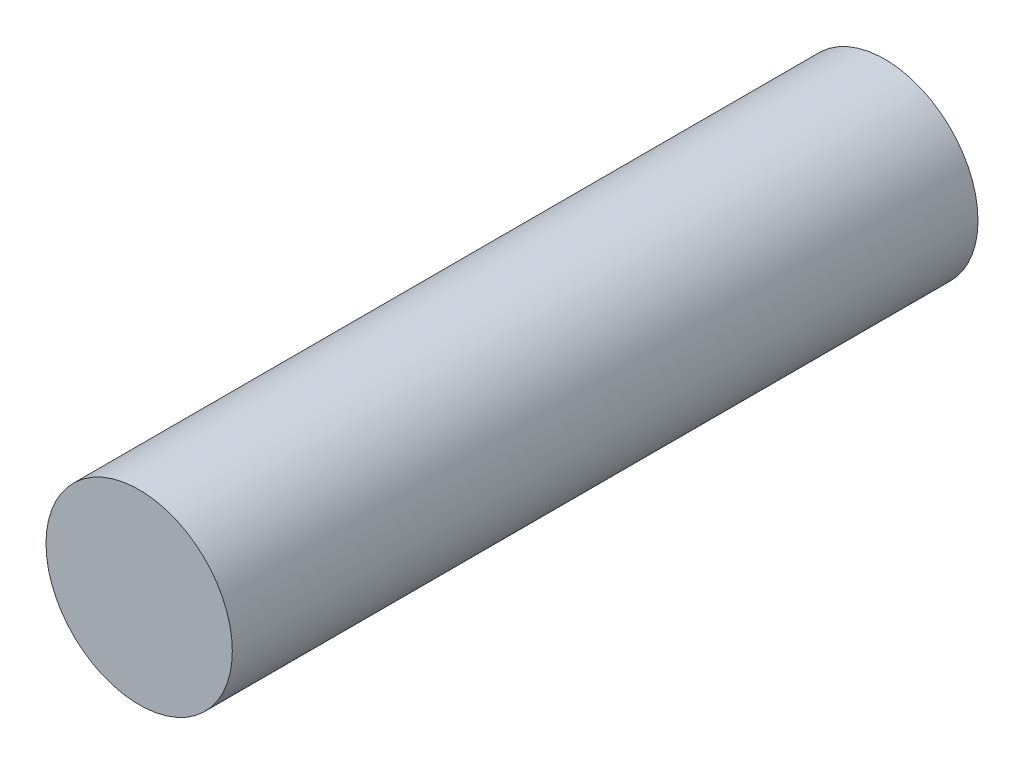
ISO-10303-21;
HEADER;
FILE_DESCRIPTION(('STEP AP214'),'2;1');
FILE_NAME('part.step','',(''),(''),'','','');
FILE_SCHEMA(('AUTOMOTIVE_DESIGN { 1 0 10303 214 1 1 1 1 }'));
ENDSEC;
DATA;
#1=APPLICATION_CONTEXT('core data for automotive mechanical design processes');
#2=APPLICATION_PROTOCOL_DEFINITION('international standard','automotive_design',2000,#1);
#3=PRODUCT_CONTEXT('',#1,'mechanical');
#4=PRODUCT('Part','Part','',(#3));
#5=PRODUCT_RELATED_PRODUCT_CATEGORY('part','',(#4));
#6=PRODUCT_DEFINITION_FORMATION('','',#4);
#7=PRODUCT_DEFINITION_CONTEXT('part definition',#1,'design');
#8=PRODUCT_DEFINITION('design','',#6,#7);
#9=PRODUCT_DEFINITION_SHAPE('','',#8);
#10=(LENGTH_UNIT() NAMED_UNIT(*) SI_UNIT(.MILLI.,.METRE.));
#11=(NAMED_UNIT(*) PLANE_ANGLE_UNIT() SI_UNIT($,.RADIAN.));
#12=(NAMED_UNIT(*) SI_UNIT($,.STERADIAN.) SOLID_ANGLE_UNIT());
#13=UNCERTAINTY_MEASURE_WITH_UNIT(LENGTH_MEASURE(1.E-05),#10,'distance_accuracy_value','');
#14=(GEOMETRIC_REPRESENTATION_CONTEXT(3) GLOBAL_UNCERTAINTY_ASSIGNED_CONTEXT((#13)) GLOBAL_UNIT_ASSIGNED_CONTEXT((#10,
#11,#12)) REPRESENTATION_CONTEXT('',''));
#15=CARTESIAN_POINT('',(0.,0.,0.));
#16=DIRECTION('',(0.,0.,1.));
#17=DIRECTION('',(1.,0.,0.));
#18=AXIS2_PLACEMENT_3D('',#15,#16,#17);
#19=CARTESIAN_POINT('',(0.,0.,38.1));
#20=DIRECTION('',(0.,0.,-1.));
#21=DIRECTION('',(-1.,0.,0.));
#22=AXIS2_PLACEMENT_3D('',#19,#20,#21);
#23=CYLINDRICAL_SURFACE('',#22,4.76);
#24=CARTESIAN_POINT('',(0.,0.,38.1));
#25=DIRECTION('',(0.,0.,1.));
#26=DIRECTION('',(1.,0.,0.));
#27=AXIS2_PLACEMENT_3D('',#24,#25,#26);
#28=CIRCLE('',#27,4.76);
#29=CARTESIAN_POINT('',(-4.76,0.,38.1));
#30=VERTEX_POINT('',#29);
#31=EDGE_CURVE('E10',#30,#30,#28,.T.);
#32=CARTESIAN_POINT('',(0.,0.,0.));
#33=DIRECTION('',(0.,0.,1.));
#34=DIRECTION('',(1.,0.,0.));
#35=AXIS2_PLACEMENT_3D('',#32,#33,#34);
#36=CIRCLE('',#35,4.76);
#37=CARTESIAN_POINT('',(-4.76,0.,0.));
#38=VERTEX_POINT('',#37);
#39=EDGE_CURVE('E42',#38,#38,#36,.T.);
#40=CARTESIAN_POINT('',(-4.76,0.,38.1));
#41=CARTESIAN_POINT('',(-4.76,0.,37.703125));
#42=CARTESIAN_POINT('',(-4.76,0.,37.30625));
#43=CARTESIAN_POINT('',(-4.76,0.,36.5125));
#44=CARTESIAN_POINT('',(-4.76,0.,36.115625));
#45=CARTESIAN_POINT('',(-4.76,0.,35.321875));
#46=CARTESIAN_POINT('',(-4.76,0.,34.925));
#47=CARTESIAN_POINT('',(-4.76,0.,34.13125));
#48=CARTESIAN_POINT('',(-4.76,0.,33.734375));
#49=CARTESIAN_POINT('',(-4.76,0.,32.940625));
#50=CARTESIAN_POINT('',(-4.76,0.,32.54375));
#51=CARTESIAN_POINT('',(-4.76,0.,31.75));
#52=CARTESIAN_POINT('',(-4.76,0.,31.353125));
#53=CARTESIAN_POINT('',(-4.76,0.,30.559375));
#54=CARTESIAN_POINT('',(-4.76,0.,30.1625));
#55=CARTESIAN_POINT('',(-4.76,0.,29.36875));
#56=CARTESIAN_POINT('',(-4.76,0.,28.971875));
#57=CARTESIAN_POINT('',(-4.76,0.,28.178125));
#58=CARTESIAN_POINT('',(-4.76,0.,27.78125));
#59=CARTESIAN_POINT('',(-4.76,0.,26.9875));
#60=CARTESIAN_POINT('',(-4.76,0.,26.590625));
#61=CARTESIAN_POINT('',(-4.76,0.,25.796875));
#62=CARTESIAN_POINT('',(-4.76,0.,25.4));
#63=CARTESIAN_POINT('',(-4.76,0.,24.60625));
#64=CARTESIAN_POINT('',(-4.76,0.,24.209375));
#65=CARTESIAN_POINT('',(-4.76,0.,23.415625));
#66=CARTESIAN_POINT('',(-4.76,0.,23.01875));
#67=CARTESIAN_POINT('',(-4.76,0.,22.225));
#68=CARTESIAN_POINT('',(-4.76,0.,21.828125));
#69=CARTESIAN_POINT('',(-4.76,0.,21.034375));
#70=CARTESIAN_POINT('',(-4.76,0.,20.6375));
#71=CARTESIAN_POINT('',(-4.76,0.,19.84375));
#72=CARTESIAN_POINT('',(-4.76,0.,19.446875));
#73=CARTESIAN_POINT('',(-4.76,0.,18.653125));
#74=CARTESIAN_POINT('',(-4.76,0.,18.25625));
#75=CARTESIAN_POINT('',(-4.76,0.,17.4625));
#76=CARTESIAN_POINT('',(-4.76,0.,17.065625));
#77=CARTESIAN_POINT('',(-4.76,0.,16.271875));
#78=CARTESIAN_POINT('',(-4.76,0.,15.875));
#79=CARTESIAN_POINT('',(-4.76,0.,15.08125));
#80=CARTESIAN_POINT('',(-4.76,0.,14.684375));
#81=CARTESIAN_POINT('',(-4.76,0.,13.890625));
#82=CARTESIAN_POINT('',(-4.76,0.,13.49375));
#83=CARTESIAN_POINT('',(-4.76,0.,12.7));
#84=CARTESIAN_POINT('',(-4.76,0.,12.303125));
#85=CARTESIAN_POINT('',(-4.76,0.,11.509375));
#86=CARTESIAN_POINT('',(-4.76,0.,11.1125));
#87=CARTESIAN_POINT('',(-4.76,0.,10.31875));
#88=CARTESIAN_POINT('',(-4.76,0.,9.92187499999999));
#89=CARTESIAN_POINT('',(-4.76,0.,9.128125));
#90=CARTESIAN_POINT('',(-4.76,0.,8.73124999999999));
#91=CARTESIAN_POINT('',(-4.76,0.,7.93749999999999));
#92=CARTESIAN_POINT('',(-4.76,0.,7.54062499999999));
#93=CARTESIAN_POINT('',(-4.76,0.,6.746875));
#94=CARTESIAN_POINT('',(-4.76,0.,6.35));
#95=CARTESIAN_POINT('',(-4.76,0.,5.55625));
#96=CARTESIAN_POINT('',(-4.76,0.,5.159375));
#97=CARTESIAN_POINT('',(-4.76,0.,4.365625));
#98=CARTESIAN_POINT('',(-4.76,0.,3.96875));
#99=CARTESIAN_POINT('',(-4.76,0.,3.175));
#100=CARTESIAN_POINT('',(-4.76,0.,2.778125));
#101=CARTESIAN_POINT('',(-4.76,0.,1.984375));
#102=CARTESIAN_POINT('',(-4.76,0.,1.5875));
#103=CARTESIAN_POINT('',(-4.76,0.,0.79375));
#104=CARTESIAN_POINT('',(-4.76,0.,0.396875));
#105=CARTESIAN_POINT('',(-4.76,0.,0.));
#106=B_SPLINE_CURVE_WITH_KNOTS('',3,(#40,#41,#42,#43,#44,#45,#46,#47,#48,#49,#50,#51,#52,#53,
#54,#55,#56,#57,#58,#59,#60,#61,#62,#63,#64,#65,#66,#67,#68,#69,#70,#71,#72,#73,#74,#75,#76,#77,
#78,#79,#80,#81,#82,#83,#84,#85,#86,#87,#88,#89,#90,#91,#92,#93,#94,#95,#96,#97,#98,#99,#100,
#101,#102,#103,#104,#105),.UNSPECIFIED.,.F.,.F.,(4,2,2,2,2,2,2,2,2,2,2,2,2,2,2,2,2,2,2,2,2,2,2,
2,2,2,2,2,2,2,2,2,4),(0.,1.190625,2.38125,3.571875,4.7625,5.953125,7.14375,8.334375,
9.52500000000001,10.715625,11.90625,13.096875,14.2875,15.478125,16.66875,17.859375,19.05,
20.240625,21.43125,22.621875,23.8125,25.003125,26.19375,27.384375,28.575,29.765625,30.95625,
32.146875,33.3375,34.528125,35.71875,36.909375,38.1),.UNSPECIFIED.);
#107=EDGE_CURVE('BSEAM41',#30,#38,#106,.T.);
#108=ORIENTED_EDGE('',*,*,#31,.F.);
#109=ORIENTED_EDGE('',*,*,#39,.T.);
#110=ORIENTED_EDGE('',*,*,#107,.T.);
#111=ORIENTED_EDGE('',*,*,#107,.F.);
#112=EDGE_LOOP('',(#108,#110,#109,#111));
#113=FACE_BOUND('',#112,.T.);
#114=ADVANCED_FACE('F41',(#113),#23,.T.);
#115=CARTESIAN_POINT('',(0.,0.,38.1));
#116=DIRECTION('',(0.,0.,1.));
#117=DIRECTION('',(1.,0.,0.));
#118=AXIS2_PLACEMENT_3D('',#115,#116,#117);
#119=PLANE('',#118);
#120=ORIENTED_EDGE('',*,*,#31,.T.);
#121=EDGE_LOOP('',(#120));
#122=FACE_BOUND('',#121,.T.);
#123=ADVANCED_FACE('F57',(#122),#119,.T.);
#124=CARTESIAN_POINT('',(0.,0.,0.));
#125=DIRECTION('',(0.,0.,1.));
#126=DIRECTION('',(1.,0.,0.));
#127=AXIS2_PLACEMENT_3D('',#124,#125,#126);
#128=PLANE('',#127);
#129=ORIENTED_EDGE('',*,*,#39,.F.);
#130=EDGE_LOOP('',(#129));
#131=FACE_BOUND('',#130,.T.);
#132=ADVANCED_FACE('F53',(#131),#128,.F.);
#133=CLOSED_SHELL('',(#114,#123,#132));
#134=MANIFOLD_SOLID_BREP('B2',#133);
#135=ADVANCED_BREP_SHAPE_REPRESENTATION('',(#18,#134),#14);
#136=SHAPE_DEFINITION_REPRESENTATION(#9,#135);
ENDSEC;
END-ISO-10303-21;
